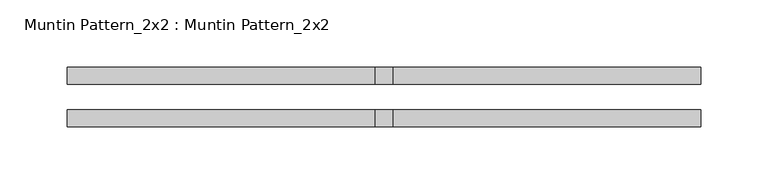
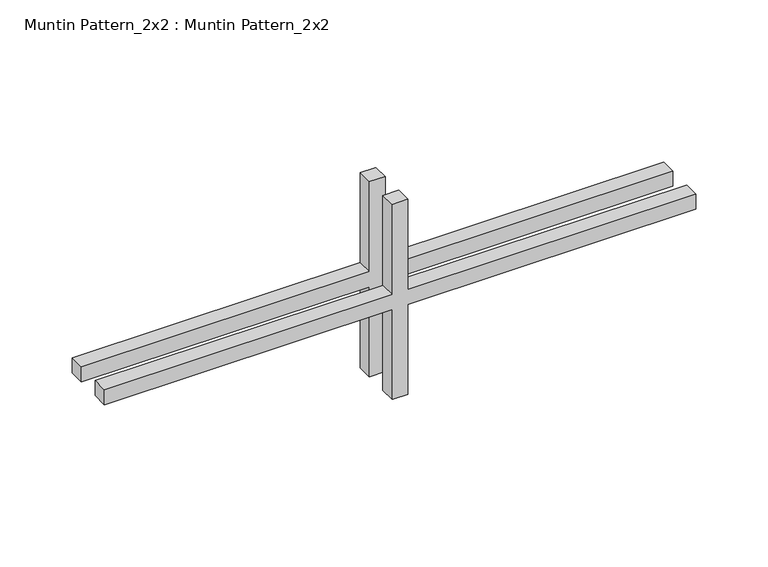
"""IFC4 building model written with IfcOpenShell, lengths in millimetres: proxy geometry, Muntin Pattern_2x2 : Muntin Pattern_2x2."""

from ifc_helpers import new_model, si_unit, frame, origin, place, context, project, spatial, polyline, outline, extrude, source, transform, mapped, element, save


def muntin_pattern_2x2_muntin_pattern_2x2_3df65231(model_context):
    return source(origin(), model_context, "Body", "SweptSolid", [
        extrude(outline(polyline([(88.9, -6.35), (88.9, -236.5375), (76.2, -236.5375), (76.2, -6.35), (0.0, -6.35), (0.0, 6.35), (76.2, 6.35), (76.2, 236.5375), (88.9, 236.5375), (88.9, 6.35), (165.1, 6.35), (165.1, -6.35), (88.9, -6.35)])), frame((0.0, -22.225, 0.0), z_axis=(0.0, 1.0, 0.0), x_axis=(0.0, 0.0, 1.0)), (0.0, 0.0, 1.0), 12.7),
        extrude(outline(polyline([(88.9, -6.35), (88.9, -236.5375), (76.2, -236.5375), (76.2, -6.35), (0.0, -6.35), (0.0, 6.35), (76.2, 6.35), (76.2, 236.5375), (88.9, 236.5375), (88.9, 6.35), (165.1, 6.35), (165.1, -6.35), (88.9, -6.35)])), frame((0.0, 9.525, 0.0), z_axis=(0.0, 1.0, 0.0), x_axis=(0.0, 0.0, 1.0)), (0.0, 0.0, 1.0), 12.7),
    ])


if __name__ == "__main__":
    model = new_model("IFC4")
    model_context = context("Model", 3, world=origin())
    ifc_project = project(units=[si_unit("LENGTHUNIT", "METRE", prefix="MILLI")], contexts=[model_context])
    site = spatial("IfcSite", under=ifc_project)
    building = spatial("IfcBuilding", under=site)
    placement = place(None, origin())
    muntin_pattern_2x2_muntin_pattern_2x2_shape = muntin_pattern_2x2_muntin_pattern_2x2_3df65231(model_context)
    element("IfcBuildingElementProxy", 1, Name="Muntin Pattern_2x2 : Muntin Pattern_2x2", ObjectType="Muntin Pattern_2x2 : Muntin Pattern_2x2", at=placement, inside=building, context=model_context, shape_type="MappedRepresentation", body=[
        mapped(muntin_pattern_2x2_muntin_pattern_2x2_shape, transform((0.0, 0.0, 0.0), x_axis=(1.0, 0.0, 0.0), y_axis=(0.0, 1.0, 0.0), z_axis=(0.0, 0.0, 1.0))),
    ])
    save(model, "model.ifc")

# Revit data of these elements
# Type "Muntin Pattern_2x2 : Muntin Pattern_2x2"
#   Width [instance default] = 4' - 0"
#   Thickness = 0' - 0 1/2"
#   Height [instance default] = 4' - 0"
#   Distance = 0' - 0 3/4"
#   Interior Material [instance default] = none
#   Exterior Material [instance default] = none
#   Default Elevation = 0
# Element 1 (IfcBuildingElementProxy, "Muntin Pattern_2x2 : Muntin Pattern_2x2")
#   Width = 1' - 6 5/8"
#   Height = 0' - 6 1/2"
#   Interior Material = Wood - Stained
#   Exterior Material = Clad - White
#   Materials on its faces: "Clad - White", "Wood - Stained"
# Materials
#   "Clad - White": class "Wood", colour RGB 242 242 238, transparency 0, Cost = 0
#   "Wood - Stained": class "Wood", colour RGB 224 178 126, transparency 0, Cost = 0
